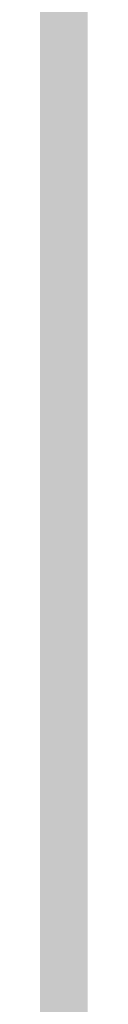
# Model space of a CAD drawing. Units: inches. Extents: x 2083 to 3317, y 1141 to 2115.
# Tile 199 of 256: x 3126.939 to 3126.9558, y 1263.6134 to 1264.1307. Entities that reach past the tile are written whole.
import ezdxf

# ---------------------------------------------------------------- set-up
doc = ezdxf.new("R2010")
doc.units = ezdxf.units.IN
doc.layers.add('A-ANNO-DIMS', color=2, linetype='Continuous', lineweight=18)
doc.layers.add('A-WALL-PATT', color=251, linetype='Continuous', lineweight=13, true_color=0x636466)
doc.styles.get("Standard").update_dxf_attribs({"font": 'arial.ttf'})
doc.dimstyles.new('ISO-25', dxfattribs={"dimtxt": 12, "dimasz": 12, "dimexe": 1.25, "dimexo": 0.625, "dimtad": 1, "dimlunit": 3, "dimtxsty": 'Standard', "dimcen": 2.5, "dimadec": 0, "dimazin": 0, "dimtfac": 1, "dimtmove": 0, "dimatfit": 3, "dimfxl": 1, "dimarcsym": 0})

# ---------------------------------------------------------------- blocks, each defined once
blk = doc.blocks.new('*D26')
at = {"layer": 'A-ANNO-DIMS', "color": 0, "lineweight": -2, "transparency": 16777216}
for p, q in [((3088.98584, 1274.91509), (3088.98584, 1270.95196)), ((3111.24004, 1274.91509), (3111.24004, 1270.95196)), ((3076.98584, 1272.20196), (2840.26245, 1272.20196)), ((3111.24004, 1272.20196), (3088.98584, 1272.20196)), ((3123.24004, 1272.20196), (3135.24004, 1272.20196))]:
    blk.add_line(p, q, dxfattribs=at)
at = {"layer": 'A-ANNO-DIMS', "color": 0, "transparency": 16777216}
for points in [[(3076.98584, 1274.20196), (3076.98584, 1270.20196), (3088.98584, 1272.20196)], [(3123.24004, 1274.20196), (3123.24004, 1270.20196), (3111.24004, 1272.20196)]]:
    blk.add_solid(points, dxfattribs=at)
at = {"layer": 'Defpoints', "color": 0, "transparency": 16777216}
for p in [(3088.98584, 1275.54009), (3111.24004, 1275.54009), (3088.98584, 1272.20196)]:
    blk.add_point(p, dxfattribs=at)
at = {"layer": 'A-ANNO-DIMS', "color": 0, "transparency": 16777216, "insert": (2952.62415, 1279.0316), "char_height": 12, "attachment_point": 5}
blk.add_mtext('NIGHTSTAND 1\'-10 1/2" TYP.', dxfattribs=at)
blk = doc.blocks.new('*D27')
at = {"layer": 'A-ANNO-DIMS', "color": 0, "lineweight": -2, "transparency": 16777216}
for p, q in [((3114.57817, 1309.79428), (3114.57817, 1321.79428)), ((3111.86504, 1297.79428), (3115.82817, 1297.79428)), ((3114.57817, 1297.79428), (3114.57817, 1275.54009)), ((3111.86504, 1275.54009), (3115.82817, 1275.54009)), ((3114.57817, 1263.54009), (3114.57817, 1140.98859))]:
    blk.add_line(p, q, dxfattribs=at)
at = {"layer": 'A-ANNO-DIMS', "color": 0, "transparency": 16777216}
for points in [[(3112.57817, 1309.79428), (3116.57817, 1309.79428), (3114.57817, 1297.79428)], [(3112.57817, 1263.54009), (3116.57817, 1263.54009), (3114.57817, 1275.54009)]]:
    blk.add_solid(points, dxfattribs=at)
at = {"layer": 'Defpoints', "color": 0, "transparency": 16777216}
for p in [(3111.24004, 1297.79428), (3111.24004, 1275.54009), (3114.57817, 1275.54009)]:
    blk.add_point(p, dxfattribs=at)
at = {"layer": 'A-ANNO-DIMS', "color": 0, "transparency": 16777216, "insert": (3107.74853, 1196.26434), "char_height": 12, "attachment_point": 5, "rotation": 90}
blk.add_mtext('1\'-10 1/2" TYP.', dxfattribs=at)

msp = doc.modelspace()

# ---------------------------------------------------------------- hatches: boundary and pattern name
at = {"layer": 'A-WALL-PATT'}
h = msp.add_hatch(color=256, dxfattribs=at)
h.dxf.hatch_style = 1
h.paths.add_polyline_path([(3126.95978, 2020.76136), (2748.95978, 2020.76136), (2604.95978, 2020.76136), (2226.95978, 2020.76136), (2226.95978, 1702.76136), (2466.95978, 1702.76136), (2466.95978, 1582.76136), (2418.95978, 1582.76136), (2418.95978, 1477.76136), (2226.95978, 1477.76136), (2226.95978, 1263.26136), (2544.95978, 1263.26136), (2544.95978, 1411.76136), (2604.95978, 1411.76136), (2685.95978, 1411.76136), (2685.95978, 1420.76136), (2604.95978, 1420.76136), (2604.95978, 1573.76136), (2604.95978, 1702.76136), (2604.95978, 2011.76136), (2748.95978, 2011.76136), (2748.95978, 1702.76136), (2862.95978, 1702.76136), (2862.95978, 1621.76136), (2871.95978, 1621.76136), (2871.95978, 1702.76136), (2883.95978, 1702.76136), (2883.95978, 1706.93946, -0.026459), (2883.95978, 1711.76136), (2757.95978, 1711.76136), (2757.95978, 1807.76136), (2787.95978, 1807.76136), (2787.95978, 1812.26136), (2757.95978, 1812.26136), (2757.95978, 2011.76136), (2877.95978, 2011.76136), (2877.95978, 1812.26136), (2847.95978, 1812.26136), (2847.95978, 1807.76136), (2889.83574, 1807.76136), (2889.83574, 1812.26136), (2882.45978, 1812.26136), (2882.45978, 2011.76136), (3117.95978, 2011.76136), (3117.95978, 1812.26136), (2937.83574, 1812.26136), (2937.83574, 1807.76136), (2995.70978, 1807.76136), (2995.70978, 1796.11767), (3000.20978, 1796.11767), (3000.20978, 1807.76136), (3117.95978, 1807.76136), (3117.95978, 1711.76136), (3000.20978, 1711.76136), (3000.20978, 1760.11767), (2998.5727, 1760.11767, -0.020711), (2995.70978, 1760.11767), (2995.70978, 1711.76136), (2931.95978, 1711.76136), (2931.95978, 1702.76136), (3126.95978, 1702.76136)])
h.paths.add_polyline_path([(2471.45978, 2011.76136), (2471.45978, 1810.01136), (2462.71694, 1810.01136), (2462.71694, 1805.51136), (2505.95978, 1805.51136), (2505.95978, 1810.01136), (2475.95978, 1810.01136), (2475.95978, 2011.76136), (2595.95978, 2011.76136), (2595.95978, 1810.01136), (2565.95978, 1810.01136), (2565.95978, 1805.51136), (2595.95978, 1805.51136), (2595.95978, 1711.76136), (2235.95978, 1711.76136), (2235.95978, 1805.51136), (2353.70978, 1805.51136), (2353.70978, 1796.05416), (2358.20978, 1796.05416), (2358.20978, 1805.51136), (2414.71694, 1805.51136), (2414.71694, 1810.01136), (2235.95978, 1810.01136), (2235.95978, 2011.76136)], flags=16)
h.paths.add_polyline_path([(2270.20473, 1994.61001), (2270.20473, 1970.61001), (2246.20473, 1970.61001), (2246.20473, 1994.61001)], flags=0)
edge = h.paths.add_edge_path(flags=0)
edge.add_ellipse((2332.02739, 1899.79818), major_axis=(-3.04299, 3.04299), ratio=0.1682525, start_angle=-161.33217, end_angle=-156.30711, ccw=False)
edge.add_ellipse((2333.08204, 1898.74353), major_axis=(-1.05465, 1.05465), ratio=0.4535321, start_angle=-123.37102, end_angle=-94.15911)
edge = h.paths.add_edge_path(flags=0)
edge.add_ellipse((2332.02739, 1968.87629), major_axis=(3.04299, 3.04299), ratio=0.1682525, start_angle=18.66783, end_angle=23.69289)
edge.add_spline(control_points=[(2332.9256, 1970.6911), (2332.22677, 1970.3361), (2330.89371, 1969.65891), (2328.41308, 1970.93214), (2327.20393, 1967.74871), (2324.7096, 1969.95559), (2322.53282, 1967.01235), (2320.01285, 1971.29581), (2317.68031, 1968.15784), (2316.04053, 1967.10205), (2315.4269, 1966.8096)], knot_values=[0, 0, 0, 0, 2.267059, 4.324559, 6.685584, 8.878641, 11.121502, 14.300359, 17.755284, 19.732645, 19.732645, 19.732645, 19.732645], degree=3, periodic=0)
edge.add_ellipse((2332.02739, 1968.87629), major_axis=(3.04299, 3.04299), ratio=0.1682525, start_angle=18.66783, end_angle=23.69289, ccw=False)
edge.add_ellipse((2333.08204, 1969.93094), major_axis=(1.05465, 1.05465), ratio=0.4535321, start_angle=56.62898, end_angle=85.84089, ccw=False)
edge = h.paths.add_edge_path(flags=0)
edge.add_spline(control_points=[(2296.42829, 1967.98791), (2293.6278, 1965.33631), (2287.70362, 1959.72709), (2299.74386, 1949.9957), (2294.53259, 1935.66853), (2290.57323, 1920.60351), (2293.39412, 1909.97369), (2296.18541, 1904.96654)], knot_values=[0.099185, 0.099185, 0.099185, 0.099185, 0.345301, 0.619822, 0.982653, 1.386093, 1.810555, 1.810555, 1.810555, 1.810555], degree=3, periodic=0)
edge.add_spline(control_points=[(2296.18541, 1904.96654), (2297.38358, 1902.6193), (2298.00097, 1901.94931), (2298.55297, 1901.46815)], knot_values=[0.006246, 0.006246, 0.006246, 0.006246, 0.055476, 0.055476, 0.055476, 0.055476], degree=3, periodic=0)
edge.add_spline(control_points=[(2298.55297, 1901.46815), (2297.25861, 1900.92322), (2295.22529, 1900.23213), (2293.06023, 1900.61421), (2292.10142, 1900.78841), (2292.08958, 1900.79057)], knot_values=[0.312835, 0.312835, 0.312835, 0.312835, 0.40178, 0.474987, 0.475903, 0.475903, 0.475903, 0.475903], degree=3, periodic=0)
edge.add_arc((2292.79365, 1904.66411), 3.93701, 215.4209, 259.69818, ccw=False)
edge.add_spline(control_points=[(2289.58531, 1902.3823), (2289.47665, 1902.53509), (2289.36848, 1902.68804), (2289.26086, 1902.84117)], knot_values=[0.102872, 0.102872, 0.102872, 0.102872, 0.116896, 0.116896, 0.116896, 0.116896], degree=3, periodic=0)
edge.add_spline(control_points=[(2289.26086, 1902.84117), (2288.6866, 1902.55019), (2287.64005, 1902.0199), (2285.88134, 1901.87395), (2283.85297, 1901.50435), (2281.71999, 1899.71054), (2278.46699, 1899.49294), (2276.15714, 1901.8832), (2272.25895, 1899.80407), (2267.77761, 1901.84318), (2262.24388, 1900.18403), (2257.41493, 1901.78206), (2254.31837, 1900.72612), (2253.17828, 1900.33734)], knot_values=[0, 0, 0, 0, 1.907977, 3.477176, 5.261074, 7.972851, 11.680248, 13.717921, 16.939592, 22.789562, 27.502503, 33.595215, 37.145618, 37.145618, 37.145618, 37.145618], degree=3, periodic=0)
edge.add_line((2253.17828, 1900.33734), (2250.24424, 1902.84117))
edge.add_line((2250.24424, 1902.84117), (2250.24424, 1965.8333))
edge.add_line((2250.24424, 1965.8333), (2253.17828, 1968.33712))
edge.add_spline(control_points=[(2253.17828, 1968.33712), (2254.31837, 1967.94835), (2257.41493, 1966.89241), (2262.24388, 1968.49043), (2267.77761, 1966.83128), (2271.52673, 1968.53722), (2273.87591, 1967.82829), (2274.2067, 1967.72764)], knot_values=[0, 0, 0, 0, 0.09018, 0.244935, 0.364644, 0.513233, 0.537855, 0.537855, 0.537855, 0.537855], degree=3, periodic=0)
edge.add_arc((2274.35289, 1963.79335), 3.93701, 72.05113, 92.12795, ccw=False)
edge.add_arc((2281.29693, 1985.23), 18.5963, 252.051134, 288.565722)
edge.add_arc((2292.31672, 1956.02888), 12.64608, 71.026788, 113.778218, ccw=False)
edge = h.paths.add_edge_path(flags=0)
edge.add_spline(control_points=[(2274.89941, 1951.85619), (2275.06616, 1951.61659), (2275.23269, 1951.37659), (2275.39799, 1951.13585)], knot_values=[1.409916, 1.409916, 1.409916, 1.409916, 1.43159, 1.43159, 1.43159, 1.43159], degree=3, periodic=0)
edge.add_spline(control_points=[(2275.39799, 1951.13585), (2275.79211, 1950.56189), (2276.17923, 1949.98377), (2276.54555, 1949.3971)], knot_values=[1.358238, 1.358238, 1.358238, 1.358238, 1.409916, 1.409916, 1.409916, 1.409916], degree=3, periodic=0)
edge.add_line((2276.54555, 1949.3971), (2277.43729, 1947.86218))
edge.add_spline(control_points=[(2277.43729, 1947.86218), (2276.30383, 1945.67311), (2274.6397, 1942.42688), (2274.63161, 1938.0939), (2272.79912, 1930.85155), (2274.35643, 1943.89705), (2275.94768, 1947.92336), (2276.54555, 1949.3971)], knot_values=[0.005632, 0.005632, 0.005632, 0.005632, 0.186014, 0.266002, 0.357087, 0.59639, 0.739732, 0.739732, 0.739732, 0.739732], degree=3, periodic=0)
edge.add_spline(control_points=[(2276.54555, 1949.3971), (2276.17923, 1949.98377), (2275.79211, 1950.56189), (2275.39799, 1951.13585)], knot_values=[1.358238, 1.358238, 1.358238, 1.358238, 1.409916, 1.409916, 1.409916, 1.409916], degree=3, periodic=0)
edge.add_spline(control_points=[(2275.39799, 1951.13585), (2274.9425, 1950.08045), (2274.20776, 1948.02527), (2273.9346, 1944.85148), (2272.46853, 1937.62749), (2273.46622, 1945.69647), (2274.70062, 1951.05947), (2274.89941, 1951.85619)], knot_values=[0.104364, 0.104364, 0.104364, 0.104364, 0.189636, 0.269624, 0.36071, 0.600013, 0.644622, 0.644622, 0.644622, 0.644622], degree=3, periodic=0)
h.paths.add_polyline_path([(2269.16751, 1963.12757, -0.357527), (2268.17063, 1960.97637, -0.092561), (2268.17063, 1939.43632, -0.357527), (2269.16751, 1937.28512, -0.357527), (2267.01631, 1938.282, -0.164785), (2254.68558, 1938.282, -0.357527), (2252.53438, 1937.28512, -0.357527), (2253.53126, 1939.43632, -0.092561), (2253.53126, 1960.97637, -0.357527), (2252.53438, 1963.12757, -0.357527), (2254.68558, 1962.13069, -0.164785), (2267.01631, 1962.13069, -0.357527)], flags=0)
h.paths.add_polyline_path([(2248.87407, 1967.8018), (2248.87407, 1957.02771), (2249.45778, 1957.02771), (2249.45778, 1911.64676), (2248.87407, 1911.64676), (2248.87407, 1900.87267), (2246.51186, 1900.87267, 0.197327), (2244.14966, 1902.45687), (2244.14966, 1966.21759, 0.197327), (2246.51186, 1967.8018)], flags=0)
h.paths.add_polyline_path([(2269.16751, 1931.38934, -0.357527), (2268.17063, 1929.23814, -0.092561), (2268.17063, 1907.6981, -0.357527), (2269.16751, 1905.54689, -0.357527), (2267.01631, 1906.54377, -0.164785), (2254.68558, 1906.54377, -0.357527), (2252.53438, 1905.54689, -0.357527), (2253.53126, 1907.6981, -0.092561), (2253.53126, 1929.23814, -0.357527), (2252.53438, 1931.38934, -0.357527), (2254.68558, 1930.39246, -0.164785), (2267.01631, 1930.39246, -0.357527)], flags=0)
edge = h.paths.add_edge_path(flags=0)
edge.add_spline(control_points=[(2276.19686, 1906.7237), (2276.16814, 1909.02893), (2276.11405, 1913.37185), (2270.59842, 1924.92498), (2273.90517, 1919.01278), (2275.92171, 1916.26206), (2275.47457, 1912.40215), (2277.25787, 1910.38062), (2276.69604, 1908.22504), (2276.64622, 1906.81302), (2276.61782, 1906.00841)], knot_values=[0, 0, 0, 0, 8.61026, 16.221274, 18.843057, 23.804898, 27.440828, 29.356102, 31.203478, 33.650687, 33.650687, 33.650687, 33.650687], degree=3, periodic=0)
edge.add_spline(control_points=[(2276.61782, 1906.00841), (2276.62331, 1905.62414), (2276.49774, 1904.62866), (2275.44178, 1903.85473), (2274.93731, 1903.08045), (2274.85908, 1902.84117)], knot_values=[0.156488, 0.156488, 0.156488, 0.156488, 0.184398, 0.231376, 0.250598, 0.250598, 0.250598, 0.250598], degree=3, periodic=0)
edge.add_line((2274.85908, 1902.84117), (2276.50598, 1902.84117))
edge.add_spline(control_points=[(2276.50598, 1902.84117), (2276.78831, 1903.08494), (2277.66507, 1904.1252), (2278.24954, 1904.34074), (2277.65387, 1908.52739), (2278.15567, 1906.22781), (2278.10046, 1905.28595), (2278.84667, 1904.06901), (2277.85679, 1903.41495), (2277.87419, 1902.99105), (2277.90356, 1902.84117)], knot_values=[0.059574, 0.059574, 0.059574, 0.059574, 0.080753, 0.103741, 0.16972, 0.176036, 0.207137, 0.240474, 0.262341, 0.27366, 0.27366, 0.27366, 0.27366], degree=3, periodic=0)
edge.add_line((2277.90356, 1902.84117), (2280.02983, 1902.84117))
edge.add_spline(control_points=[(2280.02983, 1902.84117), (2279.88822, 1903.0884), (2279.49926, 1903.98155), (2280.15228, 1905.93935), (2278.10362, 1909.65776), (2279.76239, 1907.18529), (2280.3279, 1904.87486), (2280.48511, 1903.48959), (2281.46327, 1903.24943), (2281.75834, 1902.9365), (2281.83404, 1902.84117)], knot_values=[0.013856, 0.013856, 0.013856, 0.013856, 0.034874, 0.088867, 0.107879, 0.126738, 0.158714, 0.193757, 0.217487, 0.226722, 0.226722, 0.226722, 0.226722], degree=3, periodic=0)
edge.add_spline(control_points=[(2281.83404, 1902.84117), (2281.78753, 1902.8267), (2281.64702, 1902.78299), (2281.39553, 1902.85949), (2281.08808, 1902.98524), (2280.72068, 1903.0609), (2280.33345, 1903.02573), (2280.12477, 1902.89888), (2280.02983, 1902.84117)], knot_values=[0, 0, 0, 0, 0.14413, 0.435517, 0.749276, 1.153046, 1.548371, 1.878348, 1.878348, 1.878348, 1.878348], degree=3, periodic=0)
edge.add_line((2280.02983, 1902.84117), (2277.90356, 1902.84117))
edge.add_spline(control_points=[(2277.90356, 1902.84117), (2277.89286, 1902.79586), (2277.8654, 1902.67964), (2277.60748, 1902.68748), (2277.27405, 1902.8007), (2276.83792, 1902.61977), (2276.58381, 1902.78926), (2276.50598, 1902.84117)], knot_values=[0, 0, 0, 0, 0.127189, 0.326199, 0.628009, 1.24357, 1.515331, 1.515331, 1.515331, 1.515331], degree=3, periodic=0)
edge.add_line((2276.50598, 1902.84117), (2274.85908, 1902.84117))
edge.add_spline(control_points=[(2274.85908, 1902.84117), (2274.81444, 1902.89859), (2274.72513, 1903.01345), (2274.49348, 1903.11897), (2274.24429, 1902.96054), (2273.93712, 1903.18494), (2273.61404, 1902.98314), (2273.40832, 1902.88304), (2273.32225, 1902.84117)], knot_values=[0, 0, 0, 0, 0.21843, 0.436957, 0.687977, 0.990379, 1.398396, 1.69185, 1.69185, 1.69185, 1.69185], degree=3, periodic=0)
edge.add_spline(control_points=[(2273.32225, 1902.84117), (2273.61674, 1903.44569), (2274.274, 1904.53825), (2276.02724, 1904.5737), (2276.20696, 1906.58364), (2276.19686, 1906.7237)], knot_values=[0.012227, 0.012227, 0.012227, 0.012227, 0.059472, 0.106218, 0.134458, 0.134458, 0.134458, 0.134458], degree=3, periodic=0)
h.paths.add_polyline_path([(2270.77605, 1897.78983), (2270.77605, 1873.78983), (2246.77605, 1873.78983), (2246.77605, 1897.78983)], flags=0)
h.paths.add_polyline_path([(2353.70978, 1760.00506), (2353.70978, 1760.05416), (2358.20978, 1760.05416, -0.033729)], flags=0)
h.paths.add_polyline_path([(2321.81912, 1737.52919), (2341.99533, 1737.52919, -0.414214), (2343.20327, 1736.32124), (2343.20327, 1721.0206, -0.414214), (2341.99533, 1719.81265), (2321.81912, 1719.81265, -0.414214), (2320.61117, 1721.0206), (2320.61117, 1736.32124, -0.414214)], flags=0)
h.paths.add_polyline_path([(2324.23501, 1736.32124), (2339.57944, 1736.32124, -0.414214), (2341.99533, 1733.90535), (2341.99533, 1725.44973, -0.414214), (2339.57944, 1723.03384), (2333.68059, 1723.03384), (2333.84532, 1722.04547, -0.870646), (2335.4254, 1721.82589, -0.767327), (2333.92269, 1721.42324), (2331.29102, 1721.42324, -0.767327), (2329.78832, 1721.82589, -0.870646), (2331.3684, 1722.04547), (2331.53313, 1723.03384), (2324.23501, 1723.03384, -0.414214), (2321.81912, 1725.44973), (2321.81912, 1733.90535, -0.414214)], flags=0)
h.paths.add_polyline_path([(2570.48379, 1928.61544), (2589.68379, 1928.61544), (2590.16883, 1928.61544), (2590.16883, 1904.9934), (2570.48379, 1904.9934)], flags=0)
h.paths.add_polyline_path([(2574.44732, 1927.26382, -1), (2572.82884, 1927.26382, -1)], flags=0)
h.paths.add_polyline_path([(2573.08987, 1926.94088), (2573.92503, 1927.77604), (2574.14774, 1927.55333), (2573.31258, 1926.71817)], flags=0)
h.paths.add_polyline_path([(2578.77906, 1919.72962, -1), (2571.59166, 1919.72962, -1)], flags=0)
h.paths.add_polyline_path([(2578.38536, 1919.72962, -1), (2571.98536, 1919.72962, -1)], flags=0)
h.paths.add_polyline_path([(2331.59576, 1729.47622, -1), (2333.61795, 1729.47622, -1)], flags=0)
h.paths.add_polyline_path([(2578.03423, 1927.26382, -1), (2576.41574, 1927.26382, -1)], flags=0)
h.paths.add_polyline_path([(2576.68885, 1927.53109), (2576.91156, 1927.7538), (2577.74673, 1926.91863), (2577.52402, 1926.69592)], flags=0)
h.paths.add_polyline_path([(2578.13906, 1909.85954, -1), (2572.23166, 1909.85954, -1)], flags=0)
h.paths.add_polyline_path([(2577.74536, 1909.85954, -1), (2572.62536, 1909.85954, -1)], flags=0)
h.paths.add_polyline_path([(2583.79772, 1927.26382, -1), (2582.17923, 1927.26382, -1)], flags=0)
h.paths.add_polyline_path([(2582.71865, 1927.7538), (2583.55381, 1926.91863), (2583.3311, 1926.69592), (2582.49594, 1927.53109)], flags=0)
h.paths.add_polyline_path([(2582.49594, 1927.53109), (2582.71865, 1927.7538), (2583.55381, 1926.91863), (2583.3311, 1926.69592)], flags=0)
h.paths.add_polyline_path([(2587.73906, 1920.52962, -1), (2581.83166, 1920.52962, -1)], flags=0)
h.paths.add_polyline_path([(2587.34536, 1920.52962, -1), (2582.22536, 1920.52962, -1)], flags=0)
h.paths.add_polyline_path([(2587.38462, 1927.26382, -1), (2585.76613, 1927.26382, -1)], flags=0)
h.paths.add_polyline_path([(2586.08199, 1926.98025), (2586.91716, 1927.81541), (2587.13987, 1927.5927), (2586.3047, 1926.75754)], flags=0)
h.paths.add_polyline_path([(2588.37906, 1910.65954, -1), (2581.19166, 1910.65954, -1)], flags=0)
h.paths.add_polyline_path([(2587.98536, 1910.65954, -1), (2581.58536, 1910.65954, -1)], flags=0)
h.paths.add_polyline_path([(2417.16773, 1729.4779), (2437.34394, 1729.4779, -0.414214), (2438.55188, 1728.26995), (2438.55188, 1712.96931, -0.414214), (2437.34394, 1711.76136), (2417.16773, 1711.76136, -0.414214), (2415.95978, 1712.96931), (2415.95978, 1728.26995, -0.414214)], flags=0)
h.paths.add_polyline_path([(2419.58362, 1728.26995), (2434.92805, 1728.26995, -0.414214), (2437.34394, 1725.85406), (2437.34394, 1717.39844, -0.414214), (2434.92805, 1714.98255), (2429.0292, 1714.98255), (2429.19393, 1713.99418, -0.870646), (2430.77401, 1713.7746, -0.767327), (2429.2713, 1713.37195), (2426.63963, 1713.37195, -0.767327), (2425.13693, 1713.7746, -0.870646), (2426.71701, 1713.99418), (2426.88174, 1714.98255), (2419.58362, 1714.98255, -0.414214), (2417.16773, 1717.39844), (2417.16773, 1725.85406, -0.414214)], flags=0)
h.paths.add_polyline_path([(2419.58362, 1728.26995), (2434.92805, 1728.26995, -0.414214), (2437.34394, 1725.85406), (2437.34394, 1717.39844, -0.414214), (2434.92805, 1714.98255), (2429.0292, 1714.98255), (2428.35812, 1719.00903), (2427.55282, 1719.00903), (2426.88174, 1714.98255), (2419.58362, 1714.98255, -0.414214), (2417.16773, 1717.39844), (2417.16773, 1725.85406, -0.414214)], flags=0)
h.paths.add_polyline_path([(2426.94437, 1721.42492, -1), (2428.96656, 1721.42492, -1)], flags=0)
h.paths.add_polyline_path([(2475.95978, 1702.76136), (2595.95978, 1702.76136), (2595.95978, 1582.76136), (2475.95978, 1582.76136)], flags=16)
h.paths.add_polyline_path([(2427.95978, 1573.76136), (2595.95978, 1573.76136), (2595.95978, 1468.76136), (2595.95978, 1420.76136), (2384.45978, 1420.76136), (2384.45978, 1468.76136), (2427.95978, 1468.76136)], flags=16)
h.paths.add_polyline_path([(2379.95978, 1468.76136), (2379.95978, 1420.76136), (2235.95978, 1420.76136), (2235.95978, 1468.76136)], flags=16)
h.paths.add_polyline_path([(2317.816, 1466.69577), (2337.9922, 1466.69577, -0.414214), (2339.20015, 1465.48782), (2339.20015, 1450.18718, -0.414214), (2337.9922, 1448.97923), (2317.816, 1448.97923, -0.414214), (2316.60805, 1450.18718), (2316.60805, 1465.48782, -0.414214)], flags=0)
h.paths.add_polyline_path([(2320.23189, 1465.48782), (2335.57631, 1465.48782, -0.414214), (2337.9922, 1463.07193), (2337.9922, 1454.61631, -0.414214), (2335.57631, 1452.20042), (2329.67747, 1452.20042), (2329.84219, 1451.21205, -0.870646), (2331.42228, 1450.99247, -0.767327), (2329.91957, 1450.58983), (2327.2879, 1450.58983, -0.767327), (2325.7852, 1450.99247, -0.870646), (2327.36528, 1451.21205), (2327.53001, 1452.20042), (2320.23189, 1452.20042, -0.414214), (2317.816, 1454.61631), (2317.816, 1463.07193, -0.414214)], flags=0)
h.paths.add_polyline_path([(2320.23189, 1465.48782), (2335.57631, 1465.48782, -0.414214), (2337.9922, 1463.07193), (2337.9922, 1454.61631, -0.414214), (2335.57631, 1452.20042), (2329.67747, 1452.20042), (2329.00638, 1456.22691), (2328.20109, 1456.22691), (2327.53001, 1452.20042), (2320.23189, 1452.20042, -0.414214), (2317.816, 1454.61631), (2317.816, 1463.07193, -0.414214)], flags=0)
h.paths.add_polyline_path([(2327.59264, 1458.6428, -1), (2329.61483, 1458.6428, -1)], flags=0)
h.paths.add_polyline_path([(2244.41174, 1433.34045), (2241.92094, 1433.34045, -0.414214), (2240.01786, 1435.24354), (2240.01786, 1440.95281, -0.414211), (2241.92093, 1442.8559), (2244.41174, 1442.8559, -1.976472)], flags=0)
h.paths.add_polyline_path([(2245.35689, 1434.39754, -0.414214), (2245.35689, 1441.79881, -2.144098)], flags=0)
h.paths.add_polyline_path([(2535.95978, 1416.26136), (2535.95978, 1272.26136), (2235.95978, 1272.26136), (2235.95978, 1416.26136)], flags=16)
h.paths.add_polyline_path([(2260.11956, 1384.29284), (2260.11956, 1362.03865), (2237.86537, 1362.03865), (2237.86537, 1384.29284)], flags=0)
edge = h.paths.add_edge_path(flags=0)
edge.add_line((2318.25185, 1362.0933), (2318.1458, 1362.00097))
edge.add_ellipse((2317.44512, 1360.43104), major_axis=(2.82164, 2.82164), ratio=0.1682525, start_angle=18.66783, end_angle=20.94813, ccw=False)
edge.add_ellipse((2318.42305, 1361.40897), major_axis=(0.97793, 0.97793), ratio=0.4535321, start_angle=56.62898, end_angle=70.2262, ccw=False)
edge = h.paths.add_edge_path(flags=0)
edge.add_line((2319.10737, 1295.57108), (2319.01504, 1295.67713))
edge.add_ellipse((2317.44512, 1296.37781), major_axis=(-2.82164, 2.82164), ratio=0.1682525, start_angle=-161.33217, end_angle=-159.05187, ccw=False)
edge.add_ellipse((2318.42305, 1295.39988), major_axis=(-0.97793, 0.97793), ratio=0.4535321, start_angle=-123.37102, end_angle=-109.7738)
edge = h.paths.add_edge_path(flags=0)
edge.add_spline(control_points=[(2284.21035, 1301.17022), (2284.58069, 1300.44472), (2284.89119, 1299.89202), (2285.15955, 1299.46102)], knot_values=[0.039066, 0.039066, 0.039066, 0.039066, 0.055476, 0.055476, 0.055476, 0.055476], degree=3, periodic=0)
edge.add_line((2285.15955, 1299.46102), (2284.21035, 1301.17022))
edge = h.paths.add_edge_path(flags=0)
edge.add_line((2280.41246, 1297.29801), (2283.36999, 1297.03612))
edge.add_line((2283.36999, 1297.03612), (2286.40569, 1297.92631))
edge.add_spline(control_points=[(2286.40569, 1297.92631), (2285.30549, 1297.46312), (2284.34478, 1297.12915), (2283.36999, 1297.03612)], knot_values=[0.394369, 0.394369, 0.394369, 0.394369, 0.475903, 0.475903, 0.475903, 0.475903], degree=3, periodic=0)
edge.add_spline(control_points=[(2283.36999, 1297.03612), (2283.28139, 1297.02767), (2282.31629, 1296.95734), (2281.3125, 1297.13448), (2280.42344, 1297.29602), (2280.41246, 1297.29801)], knot_values=[0.312835, 0.312835, 0.312835, 0.312835, 0.320246, 0.393453, 0.394369, 0.394369, 0.394369, 0.394369], degree=3, periodic=0)
edge = h.paths.add_edge_path(flags=0)
edge.add_line((2284.43556, 1359.60729), (2280.44629, 1355.32805))
edge.add_line((2280.44629, 1355.32805), (2279.57999, 1351.01775))
edge.add_line((2279.57999, 1351.01775), (2282.41297, 1346.58043))
edge.add_spline(control_points=[(2282.41297, 1346.58043), (2283.15333, 1345.58924), (2284.2529, 1344.0289), (2284.80104, 1342.38717), (2284.93516, 1341.80554)], knot_values=[1.240098, 1.240098, 1.240098, 1.240098, 1.332892, 1.382712, 1.382712, 1.382712, 1.382712], degree=3, periodic=0)
edge.add_spline(control_points=[(2284.93516, 1341.80554), (2285.31911, 1340.1406), (2285.23303, 1338.4092), (2284.90994, 1336.65412)], knot_values=[1.097484, 1.097484, 1.097484, 1.097484, 1.240098, 1.240098, 1.240098, 1.240098], degree=3, periodic=0)
edge.add_spline(control_points=[(2284.90994, 1336.65412), (2284.58685, 1334.89904), (2284.02675, 1333.12027), (2283.46264, 1331.36058)], knot_values=[0.95487, 0.95487, 0.95487, 0.95487, 1.097484, 1.097484, 1.097484, 1.097484], degree=3, periodic=0)
edge.add_line((2283.46264, 1331.36058), (2281.89038, 1326.15336))
edge.add_line((2281.89038, 1326.15336), (2280.75626, 1321.05609))
edge.add_line((2280.75626, 1321.05609), (2280.2992, 1316.00198))
edge.add_line((2280.2992, 1316.00198), (2280.71593, 1310.95007))
edge.add_line((2280.71593, 1310.95007), (2282.02809, 1305.97214))
edge.add_line((2282.02809, 1305.97214), (2284.21035, 1301.17022))
edge.add_spline(control_points=[(2284.21035, 1301.17022), (2283.34073, 1302.73019), (2282.6119, 1304.33649), (2282.02809, 1305.97214)], knot_values=[0.099185, 0.099185, 0.099185, 0.099185, 0.241799, 0.241799, 0.241799, 0.241799], degree=3, periodic=0)
edge.add_spline(control_points=[(2282.02809, 1305.97214), (2281.44428, 1307.60778), (2281.00549, 1309.27276), (2280.71593, 1310.95007)], knot_values=[0.241799, 0.241799, 0.241799, 0.241799, 0.384413, 0.384413, 0.384413, 0.384413], degree=3, periodic=0)
edge.add_spline(control_points=[(2280.71593, 1310.95007), (2280.43324, 1312.58761), (2280.28939, 1314.27696), (2280.29889, 1315.96203), (2280.2992, 1316.00198)], knot_values=[0.384413, 0.384413, 0.384413, 0.384413, 0.523647, 0.527028, 0.527028, 0.527028, 0.527028], degree=3, periodic=0)
edge.add_spline(control_points=[(2280.2992, 1316.00198), (2280.31233, 1317.68696), (2280.47787, 1319.36793), (2280.75626, 1321.05609)], knot_values=[0.527028, 0.527028, 0.527028, 0.527028, 0.669642, 0.669642, 0.669642, 0.669642], degree=3, periodic=0)
edge.add_spline(control_points=[(2280.75626, 1321.05609), (2281.03465, 1322.74425), (2281.42588, 1324.43961), (2281.89038, 1326.15336)], knot_values=[0.669642, 0.669642, 0.669642, 0.669642, 0.812256, 0.812256, 0.812256, 0.812256], degree=3, periodic=0)
edge.add_spline(control_points=[(2281.89038, 1326.15336), (2282.26438, 1327.53325), (2282.78787, 1329.26181), (2283.35275, 1331.01778), (2283.46264, 1331.36058)], knot_values=[0.812256, 0.812256, 0.812256, 0.812256, 0.927087, 0.95487, 0.95487, 0.95487, 0.95487], degree=3, periodic=0)
edge.add_line((2283.46264, 1331.36058), (2284.90994, 1336.65412))
edge.add_line((2284.90994, 1336.65412), (2284.93516, 1341.80554))
edge.add_line((2284.93516, 1341.80554), (2282.41297, 1346.58043))
edge.add_spline(control_points=[(2282.41297, 1346.58043), (2281.27513, 1348.10379), (2280.07845, 1349.57032), (2279.57999, 1351.01775)], knot_values=[1.382712, 1.382712, 1.382712, 1.382712, 1.525326, 1.525326, 1.525326, 1.525326], degree=3, periodic=0)
edge.add_spline(control_points=[(2279.57999, 1351.01775), (2279.44328, 1351.41472), (2279.13631, 1352.85692), (2279.73519, 1354.29039), (2280.44629, 1355.32805)], knot_values=[1.525326, 1.525326, 1.525326, 1.525326, 1.564439, 1.667941, 1.667941, 1.667941, 1.667941], degree=3, periodic=0)
edge.add_spline(control_points=[(2280.44629, 1355.32805), (2281.42611, 1356.75784), (2282.93084, 1358.18256), (2284.43556, 1359.60729)], knot_values=[1.667941, 1.667941, 1.667941, 1.667941, 1.810555, 1.810555, 1.810555, 1.810555], degree=3, periodic=0)
edge.add_arc((2280.62307, 1348.51818), 11.72618, 71.026788, 113.778218)
edge.add_arc((2270.40489, 1375.59516), 17.24357, 252.051134, 288.565722, ccw=False)
edge.add_arc((2263.96597, 1355.71785), 3.65062, 72.05113, 92.12795)
edge.add_arc((2263.96597, 1355.71785), 3.65062, 92.12795, 177.98513)
edge.add_spline(control_points=[(2260.3176, 1355.8462), (2260.26042, 1354.22067), (2260.55128, 1350.18655), (2262.99934, 1346.76625), (2264.47274, 1344.64902)], knot_values=[1.43159, 1.43159, 1.43159, 1.43159, 1.564144, 1.770695, 1.770695, 1.770695, 1.770695], degree=3, periodic=0)
edge.add_line((2264.47274, 1344.64902), (2264.93559, 1343.98253))
edge.add_spline(control_points=[(2263.80104, 1340.24811), (2263.84324, 1340.51409), (2264.06724, 1341.75647), (2264.51269, 1343.00245), (2264.93505, 1343.98108)], knot_values=[0.53657, 0.53657, 0.53657, 0.53657, 0.559349, 0.644622, 0.644622, 0.644622, 0.644622], degree=3, periodic=0)
edge.add_spline(control_points=[(2264.93505, 1343.98108), (2265.11777, 1343.71497), (2265.29888, 1343.44791), (2265.47676, 1343.17936)], knot_values=[1.384077, 1.384077, 1.384077, 1.384077, 1.409916, 1.409916, 1.409916, 1.409916], degree=3, periodic=0)
edge.add_spline(control_points=[(2265.47676, 1343.17936), (2265.65464, 1342.91082), (2265.8293, 1342.64081), (2265.99913, 1342.36881)], knot_values=[1.358238, 1.358238, 1.358238, 1.358238, 1.384077, 1.384077, 1.384077, 1.384077], degree=3, periodic=0)
edge.add_line((2265.99913, 1342.36881), (2266.82601, 1340.94555))
edge.add_spline(control_points=[(2266.82601, 1340.94555), (2268.8944, 1337.08969), (2271.39817, 1325.843), (2270.51616, 1310.56856), (2275.91938, 1301.86061), (2277.78951, 1299.19945)], knot_values=[0.116896, 0.116896, 0.116896, 0.116896, 0.472987, 1.050969, 1.313793, 1.313793, 1.313793, 1.313793], degree=3, periodic=0)
edge.add_spline(control_points=[(2277.78951, 1299.19945), (2277.83941, 1299.12845), (2277.88943, 1299.0575), (2277.93957, 1298.98658)], knot_values=[0.109884, 0.109884, 0.109884, 0.109884, 0.116896, 0.116896, 0.116896, 0.116896], degree=3, periodic=0)
edge.add_line((2277.93957, 1298.98658), (2277.78885, 1299.19911))
edge.add_spline(control_points=[(2277.78885, 1299.19911), (2277.25658, 1298.92941), (2276.28635, 1298.4379), (2275.03935, 1298.33442), (2274.38333, 1298.2389), (2274.21525, 1298.20934)], knot_values=[33.12187, 33.12187, 33.12187, 33.12187, 35.029056, 36.598255, 37.144827, 37.144827, 37.144827, 37.144827], degree=3, periodic=0)
edge.add_line((2274.21525, 1298.20934), (2273.07315, 1297.89296))
edge.add_spline(control_points=[(2273.07315, 1297.89296), (2272.32294, 1297.57978), (2271.03915, 1296.51051), (2269.24839, 1296.22606), (2268.4231, 1296.37465)], knot_values=[26.532584, 26.532584, 26.532584, 26.532584, 29.198919, 31.839101, 31.839101, 31.839101, 31.839101], degree=3, periodic=0)
edge.add_line((2268.4231, 1296.37465), (2263.8785, 1297.45753))
edge.add_spline(control_points=[(2263.8785, 1297.45753), (2263.55608, 1297.35943), (2261.86031, 1296.83869), (2260.23878, 1297.28241), (2258.93345, 1297.51646)], knot_values=[15.919551, 15.919551, 15.919551, 15.919551, 16.939592, 21.226067, 21.226067, 21.226067, 21.226067], degree=3, periodic=0)
edge.add_line((2258.93345, 1297.51646), (2254.05523, 1297.32901))
edge.add_spline(control_points=[(2254.05523, 1297.32901), (2253.75553, 1297.29582), (2252.11368, 1297.16517), (2250.46187, 1297.54422), (2249.12969, 1297.66788)], knot_values=[5.306517, 5.306517, 5.306517, 5.306517, 6.276435, 10.613034, 10.613034, 10.613034, 10.613034], degree=3, periodic=0)
edge.add_line((2249.12969, 1297.66788), (2244.33165, 1296.87776))
edge.add_line((2244.33165, 1296.87776), (2241.61103, 1299.19945))
edge.add_line((2241.61103, 1299.19945), (2241.61103, 1357.6094))
edge.add_line((2241.61103, 1357.6094), (2244.33165, 1359.9311))
edge.add_line((2244.33165, 1359.9311), (2252.72882, 1359.54269))
edge.add_spline(control_points=[(2252.72882, 1359.54269), (2252.87094, 1359.54644), (2253.30574, 1359.54817), (2253.73984, 1359.51427), (2254.03174, 1359.48243)], knot_values=[0.233291, 0.233291, 0.233291, 0.233291, 0.244935, 0.268927, 0.268927, 0.268927, 0.268927], degree=3, periodic=0)
edge.add_line((2254.03174, 1359.48243), (2259.58719, 1359.41639))
edge.add_spline(control_points=[(2259.58719, 1359.41639), (2260.67707, 1359.6285), (2262.0732, 1359.897), (2263.52369, 1359.45928), (2263.83042, 1359.36595)], knot_values=[0.422516, 0.422516, 0.422516, 0.422516, 0.513233, 0.537855, 0.537855, 0.537855, 0.537855], degree=3, periodic=0)
edge.add_arc((2263.96597, 1355.71785), 3.65062, 72.05113, 92.12795, ccw=False)
edge.add_arc((2270.40489, 1375.59516), 17.24357, 252.051134, 288.565722)
edge.add_arc((2280.62307, 1348.51818), 11.72618, 71.026788, 113.778218, ccw=False)
h.paths.add_polyline_path([(2240.34053, 1359.43471), (2240.34053, 1349.44435), (2240.88178, 1349.44435), (2240.88178, 1307.3645), (2240.34053, 1307.3645), (2240.34053, 1297.37414), (2238.15016, 1297.37414, 0.197327), (2235.95978, 1298.84311), (2235.95978, 1357.96575, 0.197327), (2238.15016, 1359.43471)], flags=0)
h.paths.add_polyline_path([(2259.15779, 1355.1005, -0.357527), (2258.23342, 1353.10578, -0.092561), (2258.23342, 1333.1326, -0.357527), (2259.15779, 1331.13788, -0.357527), (2257.16307, 1332.06225, -0.164785), (2245.7293, 1332.06225, -0.357527), (2243.73458, 1331.13788, -0.357527), (2244.65895, 1333.1326, -0.092561), (2244.65895, 1353.10578, -0.357527), (2243.73458, 1355.1005, -0.357527), (2245.7293, 1354.17613, -0.164785), (2257.16307, 1354.17613, -0.357527)], flags=0)
edge = h.paths.add_edge_path(flags=0)
edge.add_line((2265.99913, 1342.36881), (2266.82601, 1340.94555))
edge.add_line((2266.82601, 1340.94555), (2265.30756, 1337.81407))
edge.add_line((2265.30756, 1337.81407), (2264.35823, 1334.65294))
edge.add_line((2264.35823, 1334.65294), (2264.26201, 1333.7997))
edge.add_spline(control_points=[(2264.26201, 1333.7997), (2264.20836, 1333.18705), (2264.16206, 1332.36553), (2264.00714, 1331.41393), (2263.96905, 1331.20183)], knot_values=[0.464444, 0.464444, 0.464444, 0.464444, 0.516691, 0.531608, 0.531608, 0.531608, 0.531608], degree=3, periodic=0)
edge.add_spline(control_points=[(2263.96905, 1331.20183), (2263.77453, 1330.11887), (2263.42437, 1328.79084), (2263.25742, 1328.53065), (2263.23403, 1328.51461)], knot_values=[0.372682, 0.372682, 0.372682, 0.372682, 0.44885, 0.464444, 0.464444, 0.464444, 0.464444], degree=3, periodic=0)
edge.add_spline(control_points=[(2263.23403, 1328.51461), (2263.09638, 1328.42023), (2263.13117, 1329.30148), (2263.27495, 1330.61575)], knot_values=[0.280919, 0.280919, 0.280919, 0.280919, 0.372682, 0.372682, 0.372682, 0.372682], degree=3, periodic=0)
edge.add_spline(control_points=[(2263.27495, 1330.61575), (2263.41874, 1331.93002), (2263.67152, 1333.67732), (2263.96985, 1335.31503)], knot_values=[0.189157, 0.189157, 0.189157, 0.189157, 0.280919, 0.280919, 0.280919, 0.280919], degree=3, periodic=0)
edge.add_spline(control_points=[(2263.96985, 1335.31503), (2264.1005, 1336.03219), (2264.41878, 1337.62191), (2264.75485, 1338.86443), (2264.94742, 1339.49112)], knot_values=[0.097394, 0.097394, 0.097394, 0.097394, 0.137578, 0.189157, 0.189157, 0.189157, 0.189157], degree=3, periodic=0)
edge.add_spline(control_points=[(2264.94742, 1339.49112), (2265.29002, 1340.60605), (2265.64424, 1341.494), (2265.99913, 1342.36881)], knot_values=[0.005632, 0.005632, 0.005632, 0.005632, 0.097394, 0.097394, 0.097394, 0.097394], degree=3, periodic=0)
h.paths.add_polyline_path([(2259.15779, 1325.67097, -0.357527), (2258.23342, 1323.67625, -0.092561), (2258.23342, 1303.70307, -0.357527), (2259.15779, 1301.70835, -0.357527), (2257.16307, 1302.63272, -0.164785), (2245.7293, 1302.63272, -0.357527), (2243.73458, 1301.70835, -0.357527), (2244.65895, 1303.70307, -0.092561), (2244.65895, 1323.67625, -0.357527), (2243.73458, 1325.67097, -0.357527), (2245.7293, 1324.74661, -0.164785), (2257.16307, 1324.74661, -0.357527)], flags=0)
edge = h.paths.add_edge_path(flags=0)
edge.add_spline(control_points=[(2261.70894, 1317.31142), (2261.67948, 1317.41758), (2261.76186, 1317.38853), (2262.49074, 1316.08987), (2262.96218, 1315.3009)], knot_values=[14.955861, 14.955861, 14.955861, 14.955861, 16.221274, 18.694826, 18.694826, 18.694826, 18.694826], degree=3, periodic=0)
edge.add_spline(control_points=[(2262.96218, 1315.3009), (2262.99044, 1315.25362), (2263.7021, 1314.06738), (2264.34898, 1313.12715), (2264.73005, 1312.16415)], knot_values=[18.694826, 18.694826, 18.694826, 18.694826, 18.843057, 22.433791, 22.433791, 22.433791, 22.433791], degree=3, periodic=0)
edge.add_spline(control_points=[(2264.73005, 1312.16415), (2264.87556, 1311.79644), (2265.17687, 1310.76981), (2265.14307, 1309.55926), (2265.24774, 1308.82419)], knot_values=[22.433791, 22.433791, 22.433791, 22.433791, 23.804898, 26.172756, 26.172756, 26.172756, 26.172756], degree=3, periodic=0)
edge.add_line((2265.24774, 1308.82419), (2265.85077, 1307.17189))
edge.add_spline(control_points=[(2265.85077, 1307.17189), (2266.06502, 1306.82168), (2266.38439, 1306.33225), (2266.4244, 1305.78055), (2266.42037, 1305.61122)], knot_values=[28.062562, 28.062562, 28.062562, 28.062562, 29.356102, 29.911721, 29.911721, 29.911721, 29.911721], degree=3, periodic=0)
edge.add_spline(control_points=[(2266.42037, 1305.61122), (2266.41612, 1305.43259), (2266.394, 1305.25), (2266.36478, 1305.06586)], knot_values=[29.911721, 29.911721, 29.911721, 29.911721, 30.497837, 30.497837, 30.497837, 30.497837], degree=3, periodic=0)
edge.add_line((2266.36478, 1305.06586), (2266.06615, 1302.1363))
edge.add_spline(control_points=[(2266.06615, 1302.1363), (2266.07124, 1301.77998), (2265.99808, 1301.19998), (2265.66327, 1300.75896), (2265.50891, 1300.58588)], knot_values=[0.156488, 0.156488, 0.156488, 0.156488, 0.184398, 0.203543, 0.203543, 0.203543, 0.203543], degree=3, periodic=0)
edge.add_line((2265.50891, 1300.58588), (2264.43534, 1299.19945))
edge.add_line((2264.43534, 1299.19945), (2265.96244, 1299.19945))
edge.add_line((2265.96244, 1299.19945), (2267.33599, 1301.17528))
edge.add_line((2267.33599, 1301.17528), (2267.31167, 1301.98624))
edge.add_spline(control_points=[(2267.31167, 1301.98624), (2267.26111, 1302.8624), (2267.16021, 1303.73713), (2267.27149, 1303.3259)], knot_values=[0.126229, 0.126229, 0.126229, 0.126229, 0.166617, 0.166617, 0.166617, 0.166617], degree=3, periodic=0)
edge.add_spline(control_points=[(2267.27149, 1303.3259), (2267.28003, 1303.2943), (2267.30979, 1303.17537), (2267.37345, 1302.88361), (2267.40612, 1302.68283), (2267.41793, 1302.60103)], knot_values=[0.166617, 0.166617, 0.166617, 0.166617, 0.16972, 0.176036, 0.180765, 0.180765, 0.180765, 0.180765], degree=3, periodic=0)
edge.add_spline(control_points=[(2267.74389, 1300.9875), (2267.68758, 1301.15094), (2267.48052, 1301.65666), (2267.48375, 1302.14479), (2267.41793, 1302.60103)], knot_values=[0.180765, 0.180765, 0.180765, 0.180765, 0.193767, 0.220139, 0.220139, 0.220139, 0.220139], degree=3, periodic=0)
edge.add_line((2267.41793, 1302.60103), (2267.74389, 1300.9875))
edge.add_spline(control_points=[(2267.74389, 1300.9875), (2267.83196, 1300.73188), (2267.93202, 1300.3099), (2267.55484, 1299.97452), (2267.42937, 1299.82921)], knot_values=[0.220139, 0.220139, 0.220139, 0.220139, 0.240474, 0.25489, 0.25489, 0.25489, 0.25489], degree=3, periodic=0)
edge.add_line((2267.42937, 1299.82921), (2267.25836, 1299.19945))
edge.add_line((2267.25836, 1299.19945), (2269.22996, 1299.19945))
edge.add_spline(control_points=[(2269.22996, 1299.19945), (2269.09865, 1299.42869), (2268.84277, 1300.01625), (2269.01157, 1300.91592), (2268.9468, 1301.66074)], knot_values=[0.013856, 0.013856, 0.013856, 0.013856, 0.034874, 0.067073, 0.067073, 0.067073, 0.067073], degree=3, periodic=0)
edge.add_line((2268.9468, 1301.66074), (2268.43158, 1303.60311))
edge.add_spline(control_points=[(2268.43158, 1303.60311), (2268.1756, 1304.19237), (2267.59621, 1305.2513), (2268.0407, 1304.62321), (2268.25139, 1304.28242)], knot_values=[0.090155, 0.090155, 0.090155, 0.090155, 0.107879, 0.120289, 0.120289, 0.120289, 0.120289], degree=3, periodic=0)
edge.add_spline(control_points=[(2268.25139, 1304.28242), (2268.36088, 1304.10533), (2269.05775, 1302.91798), (2269.38269, 1301.59042), (2269.52141, 1300.77593), (2269.57522, 1300.55578)], knot_values=[0.120289, 0.120289, 0.120289, 0.120289, 0.126738, 0.158714, 0.173506, 0.173506, 0.173506, 0.173506], degree=3, periodic=0)
edge.add_line((2269.57522, 1300.55578), (2270.6858, 1299.42126))
edge.add_spline(control_points=[(2270.6858, 1299.42126), (2270.76722, 1299.35725), (2270.83785, 1299.2814), (2270.90292, 1299.19945)], knot_values=[0.21816, 0.21816, 0.21816, 0.21816, 0.226722, 0.226722, 0.226722, 0.226722], degree=3, periodic=0)
edge.add_line((2270.9372, 1299.19291), (2270.90292, 1299.19945))
edge.add_spline(control_points=[(2270.90292, 1299.19945), (2270.85981, 1299.18603), (2270.72951, 1299.1455), (2270.49631, 1299.21644), (2270.27166, 1299.30832), (2270.12102, 1299.34796), (2270.06334, 1299.35956)], knot_values=[0.939174, 0.939174, 0.939174, 0.939174, 1.083304, 1.374691, 1.68845, 1.878348, 1.878348, 1.878348, 1.878348], degree=3, periodic=0)
edge.add_line((2270.06334, 1299.35956), (2269.22996, 1299.19945))
edge.add_line((2269.22996, 1299.19945), (2267.25836, 1299.19945))
edge.add_spline(control_points=[(2267.25836, 1299.19945), (2267.24843, 1299.15743), (2267.22297, 1299.04967), (2266.98382, 1299.05694), (2266.80921, 1299.11623), (2266.6769, 1299.10909), (2266.63653, 1299.10481)], knot_values=[0.757665, 0.757665, 0.757665, 0.757665, 0.884854, 1.083864, 1.385675, 1.515331, 1.515331, 1.515331, 1.515331], degree=3, periodic=0)
edge.add_spline(control_points=[(2266.63653, 1299.10481), (2266.48522, 1299.08879), (2266.23581, 1299.01712), (2266.03461, 1299.15132), (2265.96244, 1299.19945)], knot_values=[0, 0, 0, 0, 0.485905, 0.757665, 0.757665, 0.757665, 0.757665], degree=3, periodic=0)
edge.add_line((2265.96244, 1299.19945), (2264.43534, 1299.19945))
edge.add_line((2264.43534, 1299.19945), (2263.85844, 1299.36712))
edge.add_spline(control_points=[(2263.85844, 1299.36712), (2263.81894, 1299.37091), (2263.77953, 1299.38572), (2263.74013, 1299.4015)], knot_values=[0.845925, 0.845925, 0.845925, 0.845925, 0.978627, 0.978627, 0.978627, 0.978627], degree=3, periodic=0)
edge.add_line((2263.72179, 1299.39643), (2263.01031, 1299.19945))
edge.add_spline(control_points=[(2263.01031, 1299.19945), (2263.24579, 1299.68286), (2263.50603, 1300.12811), (2263.87349, 1300.40803)], knot_values=[0.012227, 0.012227, 0.012227, 0.012227, 0.052971, 0.052971, 0.052971, 0.052971], degree=3, periodic=0)
edge.add_spline(control_points=[(2263.87349, 1300.40803), (2263.93213, 1300.4527), (2264.08424, 1300.55298), (2264.25519, 1300.62422), (2264.35969, 1300.66475)], knot_values=[0.052971, 0.052971, 0.052971, 0.052971, 0.059472, 0.069086, 0.069086, 0.069086, 0.069086], degree=3, periodic=0)
edge.add_line((2264.35969, 1300.66475), (2265.1419, 1301.07777))
edge.add_line((2265.1419, 1301.07777), (2265.67581, 1302.79956))
edge.add_line((2265.67581, 1302.79956), (2265.5407, 1305.70407))
edge.add_line((2265.5407, 1305.70407), (2264.80307, 1309.32772))
edge.add_line((2264.80307, 1309.32772), (2263.04053, 1314.09179))
edge.add_spline(control_points=[(2263.04053, 1314.09179), (2262.38357, 1315.67144), (2261.79597, 1316.99775), (2261.70894, 1317.31142)], knot_values=[11.216896, 11.216896, 11.216896, 11.216896, 14.955861, 14.955861, 14.955861, 14.955861], degree=3, periodic=0)
h.paths.add_polyline_path([(2871.95978, 1416.26136), (2895.91005, 1416.26136), (2895.91005, 1420.76136), (2871.95978, 1420.76136), (2871.95978, 1501.76136), (2862.95978, 1501.76136), (2862.95978, 1420.76136), (2805.95978, 1420.76136), (2805.95978, 1411.76136), (2862.95978, 1411.76136), (2862.95978, 1263.26136), (3126.95978, 1263.26136), (3126.95978, 1411.76136), (3126.95978, 1486.76136), (2943.95978, 1486.76136), (2943.95978, 1477.76136), (2967.86031, 1477.76136), (2967.86031, 1420.76136), (2943.91005, 1420.76136), (2943.91005, 1416.26136), (3117.95978, 1416.26136), (3117.95978, 1420.76136), (2972.36031, 1420.76136), (2972.36031, 1477.76136), (3117.95978, 1477.76136), (3117.95978, 1420.76136), (3117.95978, 1272.26136), (2871.95978, 1272.26136)], flags=0)
h.paths.add_polyline_path([(2457.12563, 1485.94251), (2527.60265, 1485.94251), (2527.60265, 1537.6357), (2457.12563, 1537.6357)], flags=8)
h.paths.add_polyline_path([(2481.00506, 1609.9818), (2590.76582, 1609.9818), (2590.76582, 1682.00336), (2481.00506, 1682.00336)], flags=8)
h.paths.add_polyline_path([(2483.08502, 1729.12678), (2553.56205, 1729.12678), (2553.56205, 1780.81998), (2483.08502, 1780.81998)], flags=8)
h = msp.add_hatch(color=256, dxfattribs=at)
h.dxf.hatch_style = 1
h.paths.add_polyline_path([(3126.95978, 1486.76136), (2943.95978, 1486.76136), (2943.95978, 1477.76136), (2967.86031, 1477.76136), (2967.86031, 1420.76136), (2943.91005, 1420.76136), (2943.91005, 1416.26136), (3117.95978, 1416.26136), (3117.95978, 1420.76136), (2972.36031, 1420.76136), (2972.36031, 1477.76136), (3117.95978, 1477.76136), (3117.95978, 1420.76136), (3117.95978, 1272.26136), (2871.95978, 1272.26136), (2871.95978, 1416.26136), (2895.91005, 1416.26136), (2895.91005, 1420.76136), (2871.95978, 1420.76136), (2871.95978, 1501.76136), (2862.95978, 1501.76136), (2862.95978, 1420.76136), (2805.95978, 1420.76136), (2805.95978, 1411.76136), (2862.95978, 1411.76136), (2862.95978, 1263.26136), (3126.95978, 1263.26136), (3126.95978, 1411.76136)])

# ---------------------------------------------------------------- dimensions: what is measured, and where the dimension line sits
at = {"layer": 'A-ANNO-DIMS'}
for base, p1, p2, angle, text, picture, middle in [((3114.57817, 1275.54009), (3111.24004, 1297.79428), (3111.24004, 1275.54009), 270, '<> TYP.', '*D27', (3107.74853, 1196.26434)), ((3088.98584, 1272.20196), (3111.24004, 1275.54009), (3088.98584, 1275.54009), 180, 'NIGHTSTAND <> TYP.', '*D26', (2952.62415, 1279.0316))]:
    dim = msp.add_linear_dim(base=base, p1=p1, p2=p2, angle=angle, text=text, dimstyle='ISO-25', override={"dimdec": 1, "dimlfac": 1, "dimrnd": 0, "dimzin": 1, "dimdsep": 46, "dimlunit": 4, "dimfrac": 2}, dxfattribs=at)
    dim.commit()
    dim.dimension.update_dxf_attribs({"geometry": picture, "text_midpoint": middle})

doc.saveas('drawing.dxf')
